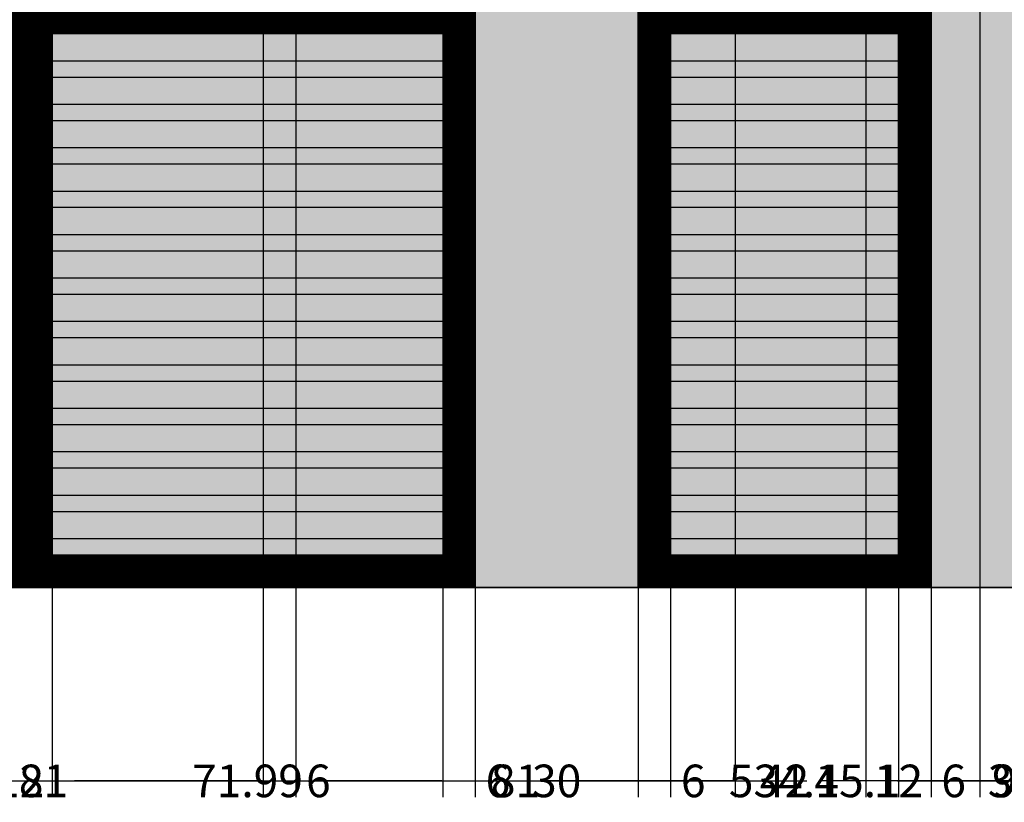
# Model space of a CAD drawing. Units: inches. Extents: x 860 to 1491, y 583 to 1370.
# Tile 2 of 8: x 1034 to 1216, y 583 to 727. Entities that reach past the tile are written whole.
import ezdxf

# ---------------------------------------------------------------- set-up
doc = ezdxf.new("R2010")
doc.units = ezdxf.units.IN
doc.header["$MEASUREMENT"] = 0
doc.layers.get('0').update_dxf_attribs({"color": 250})
for name, color, linetype, lineweight in [('A-ANNO-DIMS', 2, 'Continuous', 18), ('A-DOOR', 4, 'Continuous', 25), ('A-ELEV', 7, 'Continuous', 35), ('A-ELEV-PATT', 9, 'Continuous', 13), ('A-SITE-GATE', 3, 'Continuous', 25), ('A-SITE-PATT', 8, 'Continuous', 13), ('A-SITE-WALL', 7, 'Continuous', 35)]:
    doc.layers.add(name, color=color, linetype=linetype, lineweight=lineweight)
doc.styles.get("Standard").update_dxf_attribs({"font": 'arial.ttf'})
doc.dimstyles.get("Standard").update_dxf_attribs({"dimtxt": 6, "dimasz": 0.18, "dimexe": 3, "dimexo": 2, "dimgap": 2, "dimtad": 0, "dimtih": 1, "dimtoh": 1, "dimdec": 0, "dimzin": 0, "dimdsep": 46, "dimlunit": 3, "dimtxsty": 'Standard', "dimblk2": 'CLOSEDBLANK', "dimsah": 1, "dimcen": 2, "dimadec": 0, "dimazin": 0, "dimtfac": 1, "dimtdec": 0, "dimtofl": 0, "dimtmove": 0, "dimatfit": 3, "dimfxl": 1, "dimtolj": 1, "dimtzin": 0, "dimarcsym": 0})

# ---------------------------------------------------------------- blocks, each defined once
blk = doc.blocks.new('_ClosedBlank')
at = {"color": 0, "linetype": 'ByBlock', "lineweight": -2}
for p, q in [((-1, 0.167), (0, 0)), ((-1, 0.167), (-1, -0.167)), ((0, 0), (-1, -0.167))]:
    blk.add_line(p, q, dxfattribs=at)
blk = doc.blocks.new('*D2')
at = {"layer": 'A-ANNO-DIMS', "color": 0, "lineweight": -2, "transparency": 16777216}
for p, q in [((1442.44, 1328.76), (1442.44, 584.11)), ((908.34, 740.76), (908.34, 584.11)), ((908.52, 587.11), (1163.85, 587.11)), ((1442.26, 587.11), (1186.93, 587.11))]:
    blk.add_line(p, q, dxfattribs=at)
at = {"layer": 'A-ANNO-DIMS', "color": 0, "transparency": 16777216}
blk.add_solid([(908.52, 587.14), (908.52, 587.08), (908.34, 587.11)], dxfattribs=at)
at = {"layer": 'Defpoints', "color": 0, "transparency": 16777216}
for p in [(1442.44, 1330.76), (908.34, 742.76), (1442.44, 587.11)]:
    blk.add_point(p, dxfattribs=at)
at = {"layer": 'A-ANNO-DIMS', "color": 0, "lineweight": -2, "transparency": 16777216, "xscale": 0.18, "yscale": 0.18, "zscale": 0.18}
blk.add_blockref('_ClosedBlank', (1442.44, 587.11), dxfattribs=at)
at = {"layer": 'A-ANNO-DIMS', "color": 0, "transparency": 16777216, "insert": (1175.39, 587.11), "char_height": 6, "attachment_point": 5}
blk.add_mtext('\\A1;534.1', dxfattribs=at)
blk = doc.blocks.new('*D10')
at = {"layer": 'A-ANNO-DIMS', "color": 0, "lineweight": -2, "transparency": 16777216}
for p, q in [((1028.454444, 722.755507), (1028.454444, 584.105507)), ((1040.454446, 722.755507), (1040.454446, 584.105507)), ((1028.274444, 587.105507), (1028.094444, 587.105507)), ((1040.634446, 587.105507), (1040.814446, 587.105507))]:
    blk.add_line(p, q, dxfattribs=at)
at = {"layer": 'A-ANNO-DIMS', "color": 0, "transparency": 16777216}
blk.add_solid([(1028.274444, 587.135507), (1028.274444, 587.075507), (1028.454444, 587.105507)], dxfattribs=at)
at = {"layer": 'Defpoints', "color": 0, "transparency": 16777216}
for p in [(1028.454444, 724.755507), (1040.454446, 724.755507), (1040.454446, 587.105507)]:
    blk.add_point(p, dxfattribs=at)
at = {"layer": 'A-ANNO-DIMS', "color": 0, "lineweight": -2, "transparency": 16777216, "xscale": 0.18, "yscale": 0.18, "zscale": 0.18, "rotation": 180}
blk.add_blockref('_ClosedBlank', (1040.454446, 587.105507), dxfattribs=at)
at = {"layer": 'A-ANNO-DIMS', "color": 0, "transparency": 16777216, "insert": (1034.454445, 587.105507), "char_height": 6, "attachment_point": 5}
blk.add_mtext('\\A1;12', dxfattribs=at)
blk = doc.blocks.new('*D11')
at = {"layer": 'A-ANNO-DIMS', "color": 0, "lineweight": -2, "transparency": 16777216}
for p, q in [((1040.45, 722.76), (1040.45, 584.11)), ((1112.44, 722.76), (1112.44, 584.11)), ((1040.63, 587.11), (1064.34, 587.11)), ((1112.26, 587.11), (1088.55, 587.11))]:
    blk.add_line(p, q, dxfattribs=at)
at = {"layer": 'A-ANNO-DIMS', "color": 0, "transparency": 16777216}
blk.add_solid([(1040.63, 587.14), (1040.63, 587.08), (1040.45, 587.11)], dxfattribs=at)
at = {"layer": 'Defpoints', "color": 0, "transparency": 16777216}
for p in [(1040.45, 724.76), (1112.44, 724.76), (1112.44, 587.11)]:
    blk.add_point(p, dxfattribs=at)
at = {"layer": 'A-ANNO-DIMS', "color": 0, "lineweight": -2, "transparency": 16777216, "xscale": 0.18, "yscale": 0.18, "zscale": 0.18}
blk.add_blockref('_ClosedBlank', (1112.44, 587.11), dxfattribs=at)
at = {"layer": 'A-ANNO-DIMS', "color": 0, "transparency": 16777216, "insert": (1076.45, 587.11), "char_height": 6, "attachment_point": 5}
blk.add_mtext('\\A1;71.99', dxfattribs=at)
blk = doc.blocks.new('*D12')
at = {"layer": 'A-ANNO-DIMS', "color": 0, "lineweight": -2, "transparency": 16777216}
for p, q in [((1118.44, 740.76), (1118.44, 584.11)), ((1112.44, 722.76), (1112.44, 584.11)), ((1112.62, 587.11), (1118.26, 587.11)), ((1118.44, 587.11), (1118.62, 587.11))]:
    blk.add_line(p, q, dxfattribs=at)
at = {"layer": 'A-ANNO-DIMS', "color": 0, "transparency": 16777216}
blk.add_solid([(1112.62, 587.14), (1112.62, 587.08), (1112.44, 587.11)], dxfattribs=at)
at = {"layer": 'Defpoints', "color": 0, "transparency": 16777216}
for p in [(1118.44, 742.76), (1112.44, 724.76), (1118.44, 587.11)]:
    blk.add_point(p, dxfattribs=at)
at = {"layer": 'A-ANNO-DIMS', "color": 0, "lineweight": -2, "transparency": 16777216, "xscale": 0.18, "yscale": 0.18, "zscale": 0.18}
blk.add_blockref('_ClosedBlank', (1118.44, 587.11), dxfattribs=at)
at = {"layer": 'A-ANNO-DIMS', "color": 0, "transparency": 16777216, "insert": (1122.6, 587.11), "char_height": 6, "attachment_point": 5}
blk.add_mtext('\\A1;6', dxfattribs=at)
blk = doc.blocks.new('*D13')
at = {"layer": 'A-ANNO-DIMS', "color": 0, "lineweight": -2, "transparency": 16777216}
for p, q in [((1118.44, 740.76), (1118.44, 584.11)), ((1148.44, 740.76), (1148.44, 584.11)), ((1118.62, 587.11), (1127.16, 587.11)), ((1148.26, 587.11), (1139.73, 587.11))]:
    blk.add_line(p, q, dxfattribs=at)
at = {"layer": 'A-ANNO-DIMS', "color": 0, "transparency": 16777216}
blk.add_solid([(1118.62, 587.14), (1118.62, 587.08), (1118.44, 587.11)], dxfattribs=at)
at = {"layer": 'Defpoints', "color": 0, "transparency": 16777216}
for p in [(1118.44, 742.76), (1148.44, 742.76), (1148.44, 587.11)]:
    blk.add_point(p, dxfattribs=at)
at = {"layer": 'A-ANNO-DIMS', "color": 0, "lineweight": -2, "transparency": 16777216, "xscale": 0.18, "yscale": 0.18, "zscale": 0.18}
blk.add_blockref('_ClosedBlank', (1148.44, 587.11), dxfattribs=at)
at = {"layer": 'A-ANNO-DIMS', "color": 0, "transparency": 16777216, "insert": (1133.44, 587.11), "char_height": 6, "attachment_point": 5}
blk.add_mtext('\\A1;30', dxfattribs=at)
blk = doc.blocks.new('*D14')
at = {"layer": 'A-ANNO-DIMS', "color": 0, "lineweight": -2, "transparency": 16777216}
for p, q in [((1148.44, 740.76), (1148.44, 584.11)), ((1154.44, 722.76), (1154.44, 584.11)), ((1148.62, 587.11), (1154.26, 587.11)), ((1154.44, 587.11), (1154.62, 587.11))]:
    blk.add_line(p, q, dxfattribs=at)
at = {"layer": 'A-ANNO-DIMS', "color": 0, "transparency": 16777216}
blk.add_solid([(1148.62, 587.14), (1148.62, 587.08), (1148.44, 587.11)], dxfattribs=at)
at = {"layer": 'Defpoints', "color": 0, "transparency": 16777216}
for p in [(1148.44, 742.76), (1154.44, 724.76), (1154.44, 587.11)]:
    blk.add_point(p, dxfattribs=at)
at = {"layer": 'A-ANNO-DIMS', "color": 0, "lineweight": -2, "transparency": 16777216, "xscale": 0.18, "yscale": 0.18, "zscale": 0.18}
blk.add_blockref('_ClosedBlank', (1154.44, 587.11), dxfattribs=at)
at = {"layer": 'A-ANNO-DIMS', "color": 0, "transparency": 16777216, "insert": (1158.6, 587.11), "char_height": 6, "attachment_point": 5}
blk.add_mtext('\\A1;6', dxfattribs=at)
blk = doc.blocks.new('*D15')
at = {"layer": 'A-ANNO-DIMS', "color": 0, "lineweight": -2, "transparency": 16777216}
for p, q in [((1154.44, 722.76), (1154.44, 584.11)), ((1196.44, 722.76), (1196.44, 584.11)), ((1154.62, 587.11), (1169.05, 587.11)), ((1196.26, 587.11), (1181.83, 587.11))]:
    blk.add_line(p, q, dxfattribs=at)
at = {"layer": 'A-ANNO-DIMS', "color": 0, "transparency": 16777216}
blk.add_solid([(1154.62, 587.14), (1154.62, 587.08), (1154.44, 587.11)], dxfattribs=at)
at = {"layer": 'Defpoints', "color": 0, "transparency": 16777216}
for p in [(1154.44, 724.76), (1196.44, 724.76), (1196.44, 587.11)]:
    blk.add_point(p, dxfattribs=at)
at = {"layer": 'A-ANNO-DIMS', "color": 0, "lineweight": -2, "transparency": 16777216, "xscale": 0.18, "yscale": 0.18, "zscale": 0.18}
blk.add_blockref('_ClosedBlank', (1196.44, 587.11), dxfattribs=at)
at = {"layer": 'A-ANNO-DIMS', "color": 0, "transparency": 16777216, "insert": (1175.44, 587.11), "char_height": 6, "attachment_point": 5}
blk.add_mtext('\\A1;42', dxfattribs=at)
blk = doc.blocks.new('*D16')
at = {"layer": 'A-ANNO-DIMS', "color": 0, "lineweight": -2, "transparency": 16777216}
for p, q in [((1202.44, 740.76), (1202.44, 584.11)), ((1196.44, 722.76), (1196.44, 584.11)), ((1196.62, 587.11), (1202.26, 587.11)), ((1202.44, 587.11), (1202.62, 587.11))]:
    blk.add_line(p, q, dxfattribs=at)
at = {"layer": 'A-ANNO-DIMS', "color": 0, "transparency": 16777216}
blk.add_solid([(1196.62, 587.14), (1196.62, 587.08), (1196.44, 587.11)], dxfattribs=at)
at = {"layer": 'Defpoints', "color": 0, "transparency": 16777216}
for p in [(1202.44, 742.76), (1196.44, 724.76), (1202.44, 587.11)]:
    blk.add_point(p, dxfattribs=at)
at = {"layer": 'A-ANNO-DIMS', "color": 0, "lineweight": -2, "transparency": 16777216, "xscale": 0.18, "yscale": 0.18, "zscale": 0.18}
blk.add_blockref('_ClosedBlank', (1202.44, 587.11), dxfattribs=at)
at = {"layer": 'A-ANNO-DIMS', "color": 0, "transparency": 16777216, "insert": (1206.6, 587.11), "char_height": 6, "attachment_point": 5}
blk.add_mtext('\\A1;6', dxfattribs=at)
blk = doc.blocks.new('*D17')
at = {"layer": 'A-ANNO-DIMS', "color": 0, "lineweight": -2, "transparency": 16777216}
for p, q in [((1202.44, 740.76), (1202.44, 584.11)), ((1232.44, 740.76), (1232.44, 584.11)), ((1202.62, 587.11), (1211.16, 587.11)), ((1232.26, 587.11), (1223.73, 587.11))]:
    blk.add_line(p, q, dxfattribs=at)
at = {"layer": 'A-ANNO-DIMS', "color": 0, "transparency": 16777216}
blk.add_solid([(1202.62, 587.14), (1202.62, 587.08), (1202.44, 587.11)], dxfattribs=at)
at = {"layer": 'Defpoints', "color": 0, "transparency": 16777216}
for p in [(1202.44, 742.76), (1232.44, 742.76), (1232.44, 587.11)]:
    blk.add_point(p, dxfattribs=at)
at = {"layer": 'A-ANNO-DIMS', "color": 0, "lineweight": -2, "transparency": 16777216, "xscale": 0.18, "yscale": 0.18, "zscale": 0.18}
blk.add_blockref('_ClosedBlank', (1232.44, 587.11), dxfattribs=at)
at = {"layer": 'A-ANNO-DIMS', "color": 0, "transparency": 16777216, "insert": (1217.44, 587.11), "char_height": 6, "attachment_point": 5}
blk.add_mtext('\\A1;30', dxfattribs=at)
blk = doc.blocks.new('*D65')
at = {"layer": 'A-ANNO-DIMS', "color": 0, "lineweight": -2, "transparency": 16777216}
for p, q in [((998.34, 956.76), (998.34, 584.11)), ((1079.34, 956.76), (1079.34, 584.11)), ((998.52, 587.11), (1033.12, 587.11)), ((1079.16, 587.11), (1044.56, 587.11))]:
    blk.add_line(p, q, dxfattribs=at)
at = {"layer": 'A-ANNO-DIMS', "color": 0, "transparency": 16777216}
blk.add_solid([(998.52, 587.14), (998.52, 587.08), (998.34, 587.11)], dxfattribs=at)
at = {"layer": 'Defpoints', "color": 0, "transparency": 16777216}
for p in [(998.34, 958.76), (1079.34, 958.76), (1079.34, 587.11)]:
    blk.add_point(p, dxfattribs=at)
at = {"layer": 'A-ANNO-DIMS', "color": 0, "lineweight": -2, "transparency": 16777216, "xscale": 0.18, "yscale": 0.18, "zscale": 0.18}
blk.add_blockref('_ClosedBlank', (1079.34, 587.11), dxfattribs=at)
at = {"layer": 'A-ANNO-DIMS', "color": 0, "transparency": 16777216, "insert": (1038.84, 587.11), "char_height": 6, "attachment_point": 5}
blk.add_mtext('\\A1;81', dxfattribs=at)
blk = doc.blocks.new('*D66')
at = {"layer": 'A-ANNO-DIMS', "color": 0, "lineweight": -2, "transparency": 16777216}
for p, q in [((1079.34, 956.76), (1079.34, 584.11)), ((1085.34, 956.76), (1085.34, 584.11)), ((1079.52, 587.11), (1085.16, 587.11)), ((1085.34, 587.11), (1085.52, 587.11))]:
    blk.add_line(p, q, dxfattribs=at)
at = {"layer": 'A-ANNO-DIMS', "color": 0, "transparency": 16777216}
blk.add_solid([(1079.52, 587.14), (1079.52, 587.08), (1079.34, 587.11)], dxfattribs=at)
at = {"layer": 'Defpoints', "color": 0, "transparency": 16777216}
for p in [(1079.34, 958.76), (1085.34, 958.76), (1085.34, 587.11)]:
    blk.add_point(p, dxfattribs=at)
at = {"layer": 'A-ANNO-DIMS', "color": 0, "lineweight": -2, "transparency": 16777216, "xscale": 0.18, "yscale": 0.18, "zscale": 0.18}
blk.add_blockref('_ClosedBlank', (1085.34, 587.11), dxfattribs=at)
at = {"layer": 'A-ANNO-DIMS', "color": 0, "transparency": 16777216, "insert": (1089.5, 587.11), "char_height": 6, "attachment_point": 5}
blk.add_mtext('\\A1;6', dxfattribs=at)
blk = doc.blocks.new('*D67')
at = {"layer": 'A-ANNO-DIMS', "color": 0, "lineweight": -2, "transparency": 16777216}
for p, q in [((1085.34, 956.76), (1085.34, 584.11)), ((1166.34, 956.76), (1166.34, 584.11)), ((1085.52, 587.11), (1120.12, 587.11)), ((1166.16, 587.11), (1131.56, 587.11))]:
    blk.add_line(p, q, dxfattribs=at)
at = {"layer": 'A-ANNO-DIMS', "color": 0, "transparency": 16777216}
blk.add_solid([(1085.52, 587.14), (1085.52, 587.08), (1085.34, 587.11)], dxfattribs=at)
at = {"layer": 'Defpoints', "color": 0, "transparency": 16777216}
for p in [(1085.34, 958.76), (1166.34, 958.76), (1166.34, 587.11)]:
    blk.add_point(p, dxfattribs=at)
at = {"layer": 'A-ANNO-DIMS', "color": 0, "lineweight": -2, "transparency": 16777216, "xscale": 0.18, "yscale": 0.18, "zscale": 0.18}
blk.add_blockref('_ClosedBlank', (1166.34, 587.11), dxfattribs=at)
at = {"layer": 'A-ANNO-DIMS', "color": 0, "transparency": 16777216, "insert": (1125.84, 587.11), "char_height": 6, "attachment_point": 5}
blk.add_mtext('\\A1;81', dxfattribs=at)
blk = doc.blocks.new('*D68')
at = {"layer": 'A-ANNO-DIMS', "color": 0, "lineweight": -2, "transparency": 16777216}
for p, q in [((1211.44, 980.76), (1211.44, 584.11)), ((1166.34, 956.76), (1166.34, 584.11)), ((1166.52, 587.11), (1179.56, 587.11)), ((1211.26, 587.11), (1198.22, 587.11))]:
    blk.add_line(p, q, dxfattribs=at)
at = {"layer": 'A-ANNO-DIMS', "color": 0, "transparency": 16777216}
blk.add_solid([(1166.52, 587.14), (1166.52, 587.08), (1166.34, 587.11)], dxfattribs=at)
at = {"layer": 'Defpoints', "color": 0, "transparency": 16777216}
for p in [(1211.44, 982.76), (1166.34, 958.76), (1211.44, 587.11)]:
    blk.add_point(p, dxfattribs=at)
at = {"layer": 'A-ANNO-DIMS', "color": 0, "lineweight": -2, "transparency": 16777216, "xscale": 0.18, "yscale": 0.18, "zscale": 0.18}
blk.add_blockref('_ClosedBlank', (1211.44, 587.11), dxfattribs=at)
at = {"layer": 'A-ANNO-DIMS', "color": 0, "transparency": 16777216, "insert": (1188.89, 587.11), "char_height": 6, "attachment_point": 5}
blk.add_mtext('\\A1;45.1', dxfattribs=at)
blk = doc.blocks.new('*D69')
at = {"layer": 'A-ANNO-DIMS', "color": 0, "lineweight": -2, "transparency": 16777216}
for p, q in [((1211.440309, 980.755507), (1211.440309, 584.105507)), ((1220.440309, 896.755507), (1220.440309, 584.105507)), ((1211.260309, 587.105507), (1211.080309, 587.105507)), ((1220.620309, 587.105507), (1220.800309, 587.105507))]:
    blk.add_line(p, q, dxfattribs=at)
at = {"layer": 'A-ANNO-DIMS', "color": 0, "transparency": 16777216}
blk.add_solid([(1211.260309, 587.135507), (1211.260309, 587.075507), (1211.440309, 587.105507)], dxfattribs=at)
at = {"layer": 'Defpoints', "color": 0, "transparency": 16777216}
for p in [(1211.440309, 982.755507), (1220.440309, 898.755507), (1220.440309, 587.105507)]:
    blk.add_point(p, dxfattribs=at)
at = {"layer": 'A-ANNO-DIMS', "color": 0, "lineweight": -2, "transparency": 16777216, "xscale": 0.18, "yscale": 0.18, "zscale": 0.18, "rotation": 180}
blk.add_blockref('_ClosedBlank', (1220.440309, 587.105507), dxfattribs=at)
at = {"layer": 'A-ANNO-DIMS', "color": 0, "transparency": 16777216, "insert": (1215.940309, 587.105507), "char_height": 6, "attachment_point": 5}
blk.add_mtext('\\A1;9', dxfattribs=at)
blk = doc.blocks.new('*D76')
at = {"layer": 'A-ANNO-DIMS', "color": 0, "lineweight": -2, "transparency": 16777216}
for p, q in [((1202.440309, 1277.755507), (1202.440309, 584.105507)), ((1190.440309, 1214.755507), (1190.440309, 584.105507)), ((1190.260309, 587.105507), (1190.080309, 587.105507)), ((1202.620309, 587.105507), (1202.800309, 587.105507))]:
    blk.add_line(p, q, dxfattribs=at)
at = {"layer": 'A-ANNO-DIMS', "color": 0, "transparency": 16777216}
blk.add_solid([(1190.260309, 587.135507), (1190.260309, 587.075507), (1190.440309, 587.105507)], dxfattribs=at)
at = {"layer": 'Defpoints', "color": 0, "transparency": 16777216}
for p in [(1202.440309, 1279.755507), (1190.440309, 1216.755507), (1202.440309, 587.105507)]:
    blk.add_point(p, dxfattribs=at)
at = {"layer": 'A-ANNO-DIMS', "color": 0, "lineweight": -2, "transparency": 16777216, "xscale": 0.18, "yscale": 0.18, "zscale": 0.18, "rotation": 180}
blk.add_blockref('_ClosedBlank', (1202.440309, 587.105507), dxfattribs=at)
at = {"layer": 'A-ANNO-DIMS', "color": 0, "transparency": 16777216, "insert": (1196.440309, 587.105507), "char_height": 6, "attachment_point": 5}
blk.add_mtext('\\A1;12', dxfattribs=at)
blk = doc.blocks.new('*D77')
at = {"layer": 'A-ANNO-DIMS', "color": 0, "lineweight": -2, "transparency": 16777216}
for p, q in [((1202.44, 1277.76), (1202.44, 584.11)), ((1352.44, 1277.76), (1352.44, 584.11)), ((1202.62, 587.11), (1269.1, 587.11)), ((1352.26, 587.11), (1285.78, 587.11))]:
    blk.add_line(p, q, dxfattribs=at)
at = {"layer": 'A-ANNO-DIMS', "color": 0, "transparency": 16777216}
blk.add_solid([(1202.62, 587.14), (1202.62, 587.08), (1202.44, 587.11)], dxfattribs=at)
at = {"layer": 'Defpoints', "color": 0, "transparency": 16777216}
for p in [(1202.44, 1279.76), (1352.44, 1279.76), (1352.44, 587.11)]:
    blk.add_point(p, dxfattribs=at)
at = {"layer": 'A-ANNO-DIMS', "color": 0, "lineweight": -2, "transparency": 16777216, "xscale": 0.18, "yscale": 0.18, "zscale": 0.18}
blk.add_blockref('_ClosedBlank', (1352.44, 587.11), dxfattribs=at)
at = {"layer": 'A-ANNO-DIMS', "color": 0, "transparency": 16777216, "insert": (1277.44, 587.11), "char_height": 6, "attachment_point": 5}
blk.add_mtext('\\A1;150', dxfattribs=at)

msp = doc.modelspace()

# ---------------------------------------------------------------- hatches: boundary and pattern name
at = {"layer": 'A-ELEV-PATT'}
h = msp.add_hatch(color=256, dxfattribs=at)
h.dxf.hatch_style = 1
h.paths.add_polyline_path([(1370.4403, 730.7555), (1232.4403, 730.7555), (1232.4403, 622.7555), (1370.4403, 622.7555)])
h.paths.add_polyline_path([(1232.4403, 730.7555), (1232.4403, 742.7555), (1202.4403, 742.7555), (1202.4403, 622.7555), (1232.4403, 622.7555)])
h.paths.add_polyline_path([(1148.4403, 730.7555), (1148.4403, 742.7555), (1118.4403, 742.7555), (1118.4403, 718.7555), (1118.4403, 622.7555), (1148.4403, 622.7555)])
h.paths.add_polyline_path([(938.3403, 730.7555), (938.3403, 742.7555), (908.3403, 742.7555), (908.3403, 736.7555), (908.3403, 622.7555), (938.3403, 622.7555)])
h = msp.add_hatch(color=256, dxfattribs=at)
h.paths.add_polyline_path([(1040.4544, 724.7555), (1040.4511, 719.7555), (1112.4403, 719.7555), (1112.4403, 724.7555)])
h.paths.add_polyline_path([(1028.4511, 719.7555), (1028.4544, 724.7555), (956.3403, 724.7555), (956.3403, 719.7555)])
h.paths.add_polyline_path([(1028.4458, 711.7555), (1028.4491, 716.7555), (956.3403, 716.7555), (956.3403, 711.7555)])
h.paths.add_polyline_path([(1040.4491, 716.7555), (1040.4458, 711.7555), (1112.4403, 711.7555), (1112.4403, 716.7555)])
h.paths.add_polyline_path([(1040.4438, 708.7555), (1040.4404, 703.7555), (1112.4403, 703.7555), (1112.4403, 708.7555)])
h.paths.add_polyline_path([(1028.4351, 695.7555), (1028.4384, 700.7555), (956.3403, 700.7555), (956.3403, 695.7555)])
h.paths.add_polyline_path([(1040.4331, 692.7555), (1040.4297, 687.7555), (1112.4403, 687.7555), (1112.4403, 692.7555)])
h.paths.add_polyline_path([(1040.4224, 676.7555), (1040.419, 671.7555), (1112.4403, 671.7555), (1112.4403, 676.7555)])
h.paths.add_polyline_path([(1040.417, 668.7555), (1040.4137, 663.7555), (1112.4403, 663.7555), (1112.4403, 668.7555)])
h.paths.add_polyline_path([(1040.4063, 652.7555), (1040.403, 647.7555), (1112.4403, 647.7555), (1112.4403, 652.7555)])
h.paths.add_polyline_path([(1040.3957, 636.7555), (1040.3923, 631.7555), (1112.4403, 631.7555), (1112.4403, 636.7555)])
h = msp.add_hatch(color=256, dxfattribs=at)
h.paths.add_polyline_path([(1196.4403, 724.7555), (1154.4403, 724.7555), (1154.4403, 719.7555), (1196.4403, 719.7555)])
h.paths.add_polyline_path([(1196.4403, 716.7555), (1154.4403, 716.7555), (1154.4403, 711.7555), (1196.4403, 711.7555)])
h.paths.add_polyline_path([(1196.4403, 708.7555), (1154.4403, 708.7555), (1154.4403, 703.7555), (1196.4403, 703.7555)])
h.paths.add_polyline_path([(1196.4403, 700.7555), (1154.4403, 700.7555), (1154.4403, 695.7555), (1196.4403, 695.7555)])
h.paths.add_polyline_path([(1196.4403, 692.7555), (1154.4403, 692.7555), (1154.4403, 687.7555), (1196.4403, 687.7555)])
h.paths.add_polyline_path([(1196.4403, 684.7555), (1154.4403, 684.7555), (1154.4403, 679.7555), (1196.4403, 679.7555)])
h.paths.add_polyline_path([(1196.4403, 676.7555), (1154.4403, 676.7555), (1154.4403, 671.7555), (1196.4403, 671.7555)])
h.paths.add_polyline_path([(1196.4403, 668.7555), (1154.4403, 668.7555), (1154.4403, 663.7555), (1196.4403, 663.7555)])
h.paths.add_polyline_path([(1196.4403, 660.7555), (1154.4403, 660.7555), (1154.4403, 655.7555), (1196.4403, 655.7555)])
h.paths.add_polyline_path([(1196.4403, 652.7555), (1154.4403, 652.7555), (1154.4403, 647.7555), (1196.4403, 647.7555)])
h.paths.add_polyline_path([(1196.4403, 644.7555), (1154.4403, 644.7555), (1154.4403, 639.7555), (1196.4403, 639.7555)])
h.paths.add_polyline_path([(1196.4403, 636.7555), (1154.4403, 636.7555), (1154.4403, 631.7555), (1196.4403, 631.7555)])
h = msp.add_hatch(color=256, dxfattribs=at)
h.paths.add_polyline_path([(1028.4511, 719.7555), (956.3403, 719.7555), (956.3403, 716.7555), (1028.4491, 716.7555)])
h.paths.add_polyline_path([(1028.4458, 711.7555), (956.3403, 711.7555), (956.3403, 708.7555), (1028.4438, 708.7555)])
h.paths.add_polyline_path([(1028.4404, 703.7555), (956.3403, 703.7555), (956.3403, 700.7555), (1028.4384, 700.7555)])
h.paths.add_polyline_path([(1028.4351, 695.7555), (956.3403, 695.7555), (956.3403, 692.7555), (1028.4331, 692.7555)])
h.paths.add_polyline_path([(1028.4297, 687.7555), (956.3403, 687.7555), (956.3403, 684.7555), (1028.4277, 684.7555)])
h.paths.add_polyline_path([(1028.4244, 679.7555), (956.3403, 679.7555), (956.3403, 676.7555), (1028.4224, 676.7555)])
h.paths.add_polyline_path([(1028.419, 671.7555), (956.3403, 671.7555), (956.3403, 668.7555), (1028.417, 668.7555)])
h.paths.add_polyline_path([(1028.4137, 663.7555), (956.3403, 663.7555), (956.3403, 660.7555), (1028.4117, 660.7555)])
h.paths.add_polyline_path([(1028.4083, 655.7555), (956.3403, 655.7555), (956.3403, 652.7555), (1028.4063, 652.7555)])
h.paths.add_polyline_path([(1028.403, 647.7555), (956.3403, 647.7555), (956.3403, 644.7555), (1028.401, 644.7555)])
h.paths.add_polyline_path([(1028.3977, 639.7555), (956.3403, 639.7555), (956.3403, 636.7555), (1028.3957, 636.7555)])
h.paths.add_polyline_path([(1028.3923, 631.7555), (956.3403, 631.7555), (956.3403, 628.7555), (1028.3903, 628.7074)])
h.paths.add_polyline_path([(1112.4403, 719.7555), (1040.4511, 719.7555), (1040.4491, 716.7555), (1112.4403, 716.7555)])
h.paths.add_polyline_path([(1112.4403, 711.7555), (1040.4458, 711.7555), (1040.4438, 708.7555), (1112.4403, 708.7555)])
h.paths.add_polyline_path([(1112.4403, 703.7555), (1040.4404, 703.7555), (1040.4384, 700.7555), (1112.4403, 700.7555)])
h.paths.add_polyline_path([(1112.4403, 695.7555), (1040.4351, 695.7555), (1040.4331, 692.7555), (1112.4403, 692.7555)])
h.paths.add_polyline_path([(1112.4403, 687.7555), (1040.4297, 687.7555), (1040.4277, 684.7555), (1112.4403, 684.7555)])
h.paths.add_polyline_path([(1112.4403, 679.7555), (1040.4244, 679.7555), (1040.4224, 676.7555), (1112.4403, 676.7555)])
h.paths.add_polyline_path([(1112.4403, 671.7555), (1040.419, 671.7555), (1040.417, 668.7555), (1112.4403, 668.7555)])
h.paths.add_polyline_path([(1112.4403, 663.7555), (1040.4137, 663.7555), (1040.4117, 660.7555), (1112.4403, 660.7555)])
h.paths.add_polyline_path([(1112.4403, 655.7555), (1040.4083, 655.7555), (1040.4063, 652.7555), (1112.4403, 652.7555)])
h.paths.add_polyline_path([(1112.4403, 647.7555), (1040.403, 647.7555), (1040.401, 644.7555), (1112.4403, 644.7555)])
h.paths.add_polyline_path([(1112.4403, 639.7555), (1040.3977, 639.7555), (1040.3957, 636.7555), (1112.4403, 636.7555)])
h.paths.add_polyline_path([(1112.4403, 631.7555), (1040.3923, 631.7555), (1040.3903, 628.7555), (1112.4403, 628.7555)])
h.paths.add_polyline_path([(1196.4403, 719.7555), (1154.4403, 719.7555), (1154.4403, 716.7555), (1196.4403, 716.7555)])
h.paths.add_polyline_path([(1196.4403, 711.7555), (1154.4403, 711.7555), (1154.4403, 708.7555), (1196.4403, 708.7555)])
h.paths.add_polyline_path([(1196.4403, 703.7555), (1154.4403, 703.7555), (1154.4403, 700.7555), (1196.4403, 700.7555)])
h.paths.add_polyline_path([(1196.4403, 695.7555), (1154.4403, 695.7555), (1154.4403, 692.7555), (1196.4403, 692.7555)])
h.paths.add_polyline_path([(1196.4403, 687.7555), (1154.4403, 687.7555), (1154.4403, 684.7555), (1196.4403, 684.7555)])
h.paths.add_polyline_path([(1196.4403, 679.7555), (1154.4403, 679.7555), (1154.4403, 676.7555), (1196.4403, 676.7555)])
h.paths.add_polyline_path([(1196.4403, 671.7555), (1154.4403, 671.7555), (1154.4403, 668.7555), (1196.4403, 668.7555)])
h.paths.add_polyline_path([(1196.4403, 663.7555), (1154.4403, 663.7555), (1154.4403, 660.7555), (1196.4403, 660.7555)])
h.paths.add_polyline_path([(1196.4403, 655.7555), (1154.4403, 655.7555), (1154.4403, 652.7555), (1196.4403, 652.7555)])
h.paths.add_polyline_path([(1196.4403, 647.7555), (1154.4403, 647.7555), (1154.4403, 644.7555), (1196.4403, 644.7555)])
h.paths.add_polyline_path([(1196.4403, 639.7555), (1154.4403, 639.7555), (1154.4403, 636.7555), (1196.4403, 636.7555)])
h.paths.add_polyline_path([(1196.4403, 631.7555), (1154.4403, 631.7555), (1154.4403, 628.7555), (1196.4403, 628.7555)])
h = msp.add_hatch(color=256, dxfattribs=at)
h.paths.add_polyline_path([(1028.4438, 708.7555), (956.3403, 708.7555), (956.3403, 703.7555), (1028.4404, 703.7555)])
h.paths.add_polyline_path([(1028.4331, 692.7555), (956.3403, 692.7555), (956.3403, 687.7555), (1028.4297, 687.7555)])
h.paths.add_polyline_path([(1028.4277, 684.7555), (956.3403, 684.7555), (956.3403, 679.7555), (1028.4244, 679.7555)])
h.paths.add_polyline_path([(1028.4224, 676.7555), (956.3403, 676.7555), (956.3403, 671.7555), (1028.419, 671.7555)])
h.paths.add_polyline_path([(1028.417, 668.7555), (956.3403, 668.7555), (956.3403, 663.7555), (1028.4137, 663.7555)])
h.paths.add_polyline_path([(1028.4117, 660.7555), (956.3403, 660.7555), (956.3403, 655.7555), (1028.4083, 655.7555)])
h.paths.add_polyline_path([(1028.4063, 652.7555), (956.3403, 652.7555), (956.3403, 647.7555), (1028.403, 647.7555)])
h.paths.add_polyline_path([(1028.401, 644.7555), (956.3403, 644.7555), (956.3403, 639.7555), (1028.3977, 639.7555)])
h.paths.add_polyline_path([(1028.3957, 636.7555), (956.3403, 636.7555), (956.3403, 631.7555), (1028.3923, 631.7555)])
h.paths.add_polyline_path([(1112.4403, 644.7555), (1040.401, 644.7555), (1040.3977, 639.7555), (1112.4403, 639.7555)])
h.paths.add_polyline_path([(1112.4403, 660.7555), (1040.4117, 660.7555), (1040.4083, 655.7555), (1112.4403, 655.7555)])
h.paths.add_polyline_path([(1112.4403, 684.7555), (1040.4277, 684.7555), (1040.4244, 679.7555), (1112.4403, 679.7555)])
h.paths.add_polyline_path([(1112.4403, 700.7555), (1040.4384, 700.7555), (1040.4351, 695.7555), (1112.4403, 695.7555)])
at = {"layer": 'A-SITE-PATT'}
h = msp.add_hatch(dxfattribs=at)
h.set_pattern_fill('GRAVEL', color=256, scale=30, style=0)
h.set_pattern_definition([(228.01279, (21.6, 30), (-240, -270), [4.0361, -399.57264]), (184.96974, (18.9, 27), (360, 30), [6.92604, -685.67774]), (132.51045, (12, 26.4), (300, -330), [4.88364, -483.481]), (267.27369, (0.3, 18.9), (30, 600), [6.30714, -624.40674]), (292.83365, (0, 12.6), (-150, 360), [6.18465, -612.2812]), (357.27369, (2.4, 6.9), (-600, 30), [6.30714, -624.40674]), (37.69424, (8.7, 6.6), (-390, -300), [8.34087, -825.74546]), (72.25533, (15.3, 11.7), (210, 660), [7.87464, -779.58964]), (121.42957, (17.7, 19.2), (-240, 390), [6.3285, -626.5222]), (175.23636, (14.4, 24.6), (330, -30), [7.22496, -354.0229]), (222.39744, (7.2, 25.2), (-360, -330), [9.34344, -925.00125]), (138.81407, (30, 18.6), (-210, 180), [3.18903, -315.71534]), (171.46923, (27.6, 20.7), (390, -60), [6.0671, -600.64534]), (225, (21.6, 21.6), (-3e-15, -30), [4.24263, -38.1838]), (203.1986, (19.5, 25.2), (150, 60), [2.28474, -226.18845]), (291.8014, (17.4, 24.3), (-30, 90), [3.2311, -158.32385]), (30.96376, (18.6, 21.3), (90, 60), [5.24787, -169.6807]), (161.56505, (23.1, 24), (60, -30), [3.79473, -91.0736]), (16.38954, (0, 24.3), (300, 90), [5.316, -526.28535]), (70.34618, (5.1, 25.8), (-120, -330), [4.45983, -441.52223]), (293.1986, (23.1, 30), (-60, 150), [4.56945, -223.90374]), (343.61046, (24.9, 25.8), (-300, 90), [5.316, -526.28535]), (339.44395, (0, 5.7), (-150, 60), [5.1264, -251.1937]), (294.77514, (4.8, 3.9), (-150, 330), [4.29534, -425.2393]), (66.8014, (23.4, 0), (60, 150), [4.56945, -223.90374]), (17.35402, (25.2, 4.2), (-390, -120), [5.02893, -497.8627]), (69.44395, (8.7, 0), (-60, -150), [2.5632, -253.7569]), (101.30993, (21.6, 0), (-30, 120), [1.5297, -151.4409]), (165.96376, (21.3, 1.5), (90, -30), [6.18465, -117.5085]), (186.00901, (15.3, 3), (300, 30), [5.7315, -567.4177]), (303.69007, (18.6, 18.6), (-30, 60), [4.32666, -103.8399]), (353.15723, (21, 15), (510, -60), [7.55382, -747.82688]), (60.9454, (28.5, 14.1), (-120, -210), [3.0887, -305.7802]), (90, (30, 16.8), (-30, 30), [1.8, -28.2]), (120.25644, (14.7, 3.9), (120, -210), [4.1677, -412.6056]), (48.01279, (12.6, 7.5), (240, 270), [8.07216, -395.53656]), (0, (18, 13.5), (30, 30), [7.8, -22.2]), (325.30485, (25.8, 13.5), (300, -210), [4.7434, -469.59823]), (254.0546, (29.7, 10.8), (-30, -120), [4.36806, -214.03524]), (207.64598, (28.5, 6.6), (-570, -300), [7.11195, -704.08423]), (175.42608, (22.2, 3.3), (-390, 30), [7.52397, -744.8722])])
h.paths.add_polyline_path([(1370.4403, 730.7555), (1232.4403, 730.7555), (1232.4403, 622.7555), (1370.4403, 622.7555)])
h.paths.add_polyline_path([(1232.4403, 730.7555), (1232.4403, 742.7555), (1202.4403, 742.7555), (1202.4403, 622.7555), (1232.4403, 622.7555)])
h.paths.add_polyline_path([(1148.4403, 730.7555), (1148.4403, 742.7555), (1118.4403, 742.7555), (1118.4403, 718.7555), (1118.4403, 622.7555), (1148.4403, 622.7555)])
h.paths.add_polyline_path([(938.3403, 730.7555), (938.3403, 742.7555), (908.3403, 742.7555), (908.3403, 736.7555), (908.3403, 622.7555), (938.3403, 622.7555)])
h = msp.add_hatch(dxfattribs=at)
h.set_pattern_fill('ANSI31', color=256, style=0)
h.paths.add_polyline_path([(1118.4403, 730.7555), (962.3403, 730.7555), (950.3403, 730.7555), (950.3403, 622.7555), (1118.4403, 622.7555)])
h.paths.add_polyline_path([(1028.4544, 724.7555), (1028.3903, 628.7074), (956.3403, 628.7555), (956.3403, 724.7555)], flags=16)
h.paths.add_polyline_path([(1040.4544, 724.7555), (1112.4403, 724.7555), (1112.4403, 628.7555), (1040.3903, 628.7555)], flags=16)
h.paths.add_polyline_path([(1202.4403, 730.7555), (1148.4403, 730.7555), (1148.4403, 622.7555), (1202.4403, 622.7555)])
h.paths.add_polyline_path([(1154.4403, 724.7555), (1196.4403, 724.7555), (1196.4403, 628.7555), (1154.4403, 628.7555)], flags=16)

# ---------------------------------------------------------------- linework, layer by layer
at = {"layer": 'A-DOOR'}
msp.add_line((1118.4403, 838.7555), (1118.4403, 718.7555), dxfattribs=at)
at = {"layer": 'A-ELEV'}
msp.add_line((1202.4403, 622.7555), (1202.4403, 898.7555), dxfattribs=at)
at = {"layer": 'A-SITE-GATE'}
for p, q in [((1040.4544, 724.7555), (1040.3903, 628.7515)), ((1040.4544, 724.7555), (1112.4403, 724.7555)), ((1112.4403, 724.7555), (1112.4403, 628.7555)), ((1154.4403, 724.7555), (1154.4403, 628.7555)), ((1154.4403, 724.7555), (1196.4403, 724.7555)), ((1196.4403, 628.7555), (1196.4403, 724.7555)), ((1040.4511, 719.7555), (1112.4403, 719.7555)), ((1154.4403, 719.7555), (1196.4403, 719.7555)), ((1040.4491, 716.7555), (1112.4403, 716.7555)), ((1154.4403, 716.7555), (1196.4403, 716.7555)), ((1040.4458, 711.7555), (1112.4403, 711.7555)), ((1154.4403, 711.7555), (1196.4403, 711.7555)), ((1040.4438, 708.7555), (1112.4403, 708.7555)), ((1154.4403, 708.7555), (1196.4403, 708.7555)), ((1040.4404, 703.7555), (1112.4403, 703.7555)), ((1154.4403, 703.7555), (1196.4403, 703.7555)), ((1040.4384, 700.7555), (1112.4403, 700.7555)), ((1154.4403, 700.7555), (1196.4403, 700.7555)), ((1040.4351, 695.7555), (1112.4403, 695.7555)), ((1154.4403, 695.7555), (1196.4403, 695.7555)), ((1040.4331, 692.7555), (1112.4403, 692.7555)), ((1154.4403, 692.7555), (1196.4403, 692.7555)), ((1040.4297, 687.7555), (1112.4403, 687.7555)), ((1154.4403, 687.7555), (1196.4403, 687.7555)), ((1040.4277, 684.7555), (1112.4403, 684.7555)), ((1154.4403, 684.7555), (1196.4403, 684.7555)), ((1040.4244, 679.7555), (1112.4403, 679.7555)), ((1154.4403, 679.7555), (1196.4403, 679.7555)), ((1040.4224, 676.7555), (1112.4403, 676.7555)), ((1154.4403, 676.7555), (1196.4403, 676.7555)), ((1040.419, 671.7555), (1112.4403, 671.7555)), ((1154.4403, 671.7555), (1196.4403, 671.7555)), ((1040.417, 668.7555), (1112.4403, 668.7555)), ((1154.4403, 668.7555), (1196.4403, 668.7555)), ((1040.4137, 663.7555), (1112.4403, 663.7555)), ((1154.4403, 663.7555), (1196.4403, 663.7555)), ((1040.4117, 660.7555), (1112.4403, 660.7555)), ((1154.4403, 660.7555), (1196.4403, 660.7555)), ((1040.4083, 655.7555), (1112.4403, 655.7555)), ((1154.4403, 655.7555), (1196.4403, 655.7555)), ((1040.4063, 652.7555), (1112.4403, 652.7555)), ((1154.4403, 652.7555), (1196.4403, 652.7555)), ((1040.403, 647.7555), (1112.4403, 647.7555)), ((1154.4403, 647.7555), (1196.4403, 647.7555)), ((1040.401, 644.7555), (1112.4403, 644.7555)), ((1154.4403, 644.7555), (1196.4403, 644.7555)), ((1040.3977, 639.7555), (1112.4403, 639.7555)), ((1154.4403, 639.7555), (1196.4403, 639.7555)), ((1040.3957, 636.7555), (1112.4403, 636.7555)), ((1154.4403, 636.7555), (1196.4403, 636.7555)), ((1040.3923, 631.7555), (1112.4403, 631.7555)), ((1154.4403, 631.7555), (1196.4403, 631.7555)), ((1040.3903, 628.7555), (1112.4403, 628.7555)), ((1154.4403, 628.7555), (1196.4403, 628.7555))]:
    msp.add_line(p, q, dxfattribs=at)
at = {"layer": 'A-SITE-WALL'}
for p, q in [((1118.4403, 730.7555), (1118.4403, 622.7555)), ((1148.4403, 730.7555), (1148.4403, 622.7555)), ((908.3403, 622.7555), (1442.4403, 622.7555))]:
    msp.add_line(p, q, dxfattribs=at)

# ---------------------------------------------------------------- dimensions: what is measured, and where the dimension line sits
at = {"layer": 'A-ANNO-DIMS'}
for base, p1, p2, override, picture, middle in [((1442.4403, 587.1055), (908.3403, 742.7555), (1442.4403, 1330.7555), {"dimdec": 1, "dimlfac": 1, "dimrnd": 0, "dimzin": 0, "dimdsep": 46, "dimlunit": 2}, '*D2', (1175.3903, 587.1055)), ((1202.4403, 587.1055), (1190.4403, 1216.7555), (1202.4403, 1279.7555), {"dimdec": 0, "dimlfac": 1, "dimrnd": 0, "dimzin": 0, "dimdsep": 46, "dimlunit": 2}, '*D76', (1196.4403, 587.1055)), ((1352.4403, 587.1055), (1202.4403, 1279.7555), (1352.4403, 1279.7555), {"dimdec": 0, "dimlfac": 1, "dimrnd": 0, "dimzin": 0, "dimdsep": 46, "dimlunit": 2}, '*D77', (1277.4403, 587.1055)), ((1211.4403, 587.1055), (1166.3403, 958.7555), (1211.4403, 982.7555), {"dimdec": 1, "dimlfac": 1, "dimrnd": 0, "dimzin": 0, "dimdsep": 46, "dimlunit": 2}, '*D68', (1188.8903, 587.1055)), ((1220.4403, 587.1055), (1211.4403, 982.7555), (1220.4403, 898.7555), {"dimdec": 0, "dimlfac": 1, "dimrnd": 0, "dimzin": 0, "dimdsep": 46, "dimlunit": 2}, '*D69', (1215.9403, 587.1055)), ((1079.3403, 587.1055), (998.3403, 958.7555), (1079.3403, 958.7555), {"dimdec": 0, "dimlfac": 1, "dimrnd": 0, "dimzin": 0, "dimdsep": 46, "dimlunit": 2}, '*D65', (1038.8403, 587.1055)), ((1085.3403, 587.1055), (1079.3403, 958.7555), (1085.3403, 958.7555), {"dimdec": 0, "dimlfac": 1, "dimrnd": 0, "dimzin": 0, "dimdsep": 46, "dimlunit": 2}, '*D66', (1089.5012, 587.1055)), ((1166.3403, 587.1055), (1085.3403, 958.7555), (1166.3403, 958.7555), {"dimdec": 0, "dimlfac": 1, "dimrnd": 0, "dimzin": 0, "dimdsep": 46, "dimlunit": 2}, '*D67', (1125.8403, 587.1055)), ((1118.4403, 587.1055), (1112.4403, 724.7555), (1118.4403, 742.7555), {"dimdec": 0, "dimlfac": 1, "dimrnd": 0, "dimzin": 0, "dimdsep": 46, "dimlunit": 2}, '*D12', (1122.6012, 587.1055)), ((1148.4403, 587.1055), (1118.4403, 742.7555), (1148.4403, 742.7555), {"dimdec": 0, "dimlfac": 1, "dimrnd": 0, "dimzin": 0, "dimdsep": 46, "dimlunit": 2}, '*D13', (1133.4403, 587.1055)), ((1154.4403, 587.1055), (1148.4403, 742.7555), (1154.4403, 724.7555), {"dimdec": 0, "dimlfac": 1, "dimrnd": 0, "dimzin": 0, "dimdsep": 46, "dimlunit": 2}, '*D14', (1158.6012, 587.1055)), ((1202.4403, 587.1055), (1196.4403, 724.7555), (1202.4403, 742.7555), {"dimdec": 0, "dimlfac": 1, "dimrnd": 0, "dimzin": 0, "dimdsep": 46, "dimlunit": 2}, '*D16', (1206.6012, 587.1055)), ((1232.4403, 587.1055), (1202.4403, 742.7555), (1232.4403, 742.7555), {"dimdec": 0, "dimlfac": 1, "dimrnd": 0, "dimzin": 0, "dimdsep": 46, "dimlunit": 2}, '*D17', (1217.4403, 587.1055)), ((1040.4544, 587.1055), (1028.4544, 724.7555), (1040.4544, 724.7555), {"dimdec": 0, "dimlfac": 1, "dimrnd": 0, "dimzin": 0, "dimdsep": 46, "dimlunit": 2}, '*D10', (1034.4544, 587.1055)), ((1112.4403, 587.1055), (1040.4544, 724.7555), (1112.4403, 724.7555), {"dimdec": 2, "dimlfac": 1, "dimrnd": 0, "dimzin": 0, "dimdsep": 46, "dimlunit": 2}, '*D11', (1076.4474, 587.1055)), ((1196.4403, 587.1055), (1154.4403, 724.7555), (1196.4403, 724.7555), {"dimdec": 0, "dimlfac": 1, "dimrnd": 0, "dimzin": 0, "dimdsep": 46, "dimlunit": 2}, '*D15', (1175.4403, 587.1055))]:
    dim = msp.add_linear_dim(base=base, p1=p1, p2=p2, dimstyle='Standard', override=override, dxfattribs=at)
    dim.commit()
    dim.dimension.update_dxf_attribs({"geometry": picture, "text_midpoint": middle})

doc.saveas('drawing.dxf')
